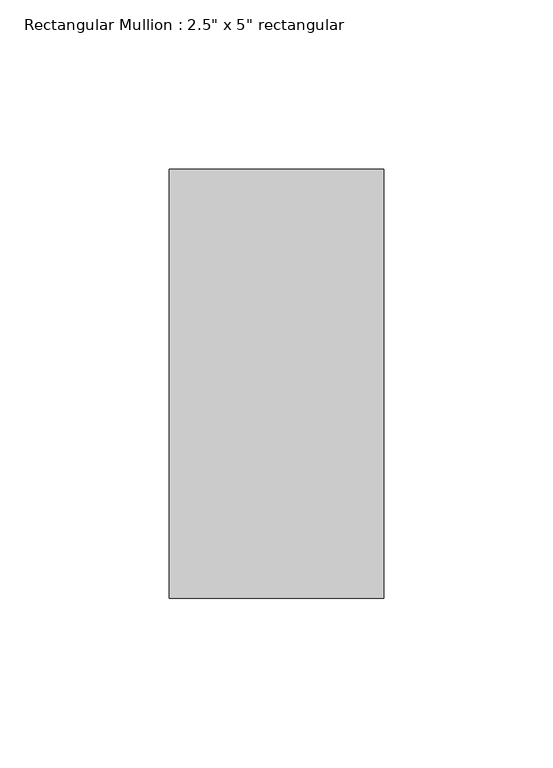
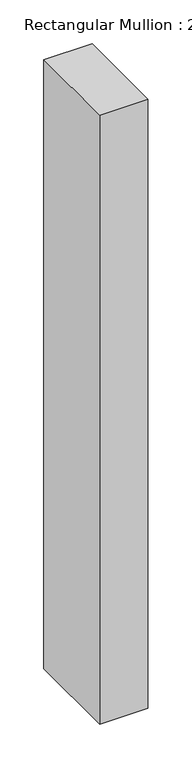
"""IFC4 building model written with IfcOpenShell, lengths in millimetres: member geometry."""

from ifc_helpers import new_model, si_unit, frame, origin, place, context, project, spatial, polyline, outline, extrude, source, transform, mapped, element, save


def member_19f58c97(model_context):
    return source(origin(), model_context, "Body", "SweptSolid", [
        extrude(outline(polyline([(0.0, 63.5), (0.0, -63.5), (-63.5, -63.5), (-63.5, 63.5), (0.0, 63.5)])), frame((0.0, 0.0, -848.0104839), z_axis=(0.0, 0.0, 1.0), x_axis=(1.0, 0.0, 0.0)), (0.0, 0.0, 1.0), 848.0104839),
    ])


if __name__ == "__main__":
    model = new_model("IFC4")
    model_context = context("Model", 3, world=origin())
    ifc_project = project(units=[si_unit("LENGTHUNIT", "METRE", prefix="MILLI")], contexts=[model_context])
    site = spatial("IfcSite", under=ifc_project)
    building = spatial("IfcBuilding", under=site)
    placement = place(None, origin())
    member_shape = member_19f58c97(model_context)
    element("IfcMember", 1, ObjectType="Rectangular Mullion : 2.5\" x 5\" rectangular", at=placement, inside=building, context=model_context, shape_type="MappedRepresentation", body=[
        mapped(member_shape, transform((0.0, 0.0, 0.0), x_axis=(1.0, 0.0, 0.0), y_axis=(0.0, 1.0, 0.0), z_axis=(0.0, 0.0, 1.0))),
    ])
    save(model, "model.ifc")

# Revit data of these elements
# Type "Rectangular Mullion : 2.5\" x 5\" rectangular"
#   built-in parameter 1007304 = 0.416667 (stored number, unit not read)
#   built-in parameter 1007301 = 0.104167 (stored number, unit not read)
#   built-in parameter 1007300 = 0.104167 (stored number, unit not read)
# Element 1 (IfcMember, "Rectangular Mullion : 2.5\" x 5\" rectangular")
#   Materials on its faces: "Aluminum"
# Materials
#   "Aluminum": class "Metal", colour RGB 247 247 247, transparency 0, Description = "Aluminum 6061", Cost = 0
